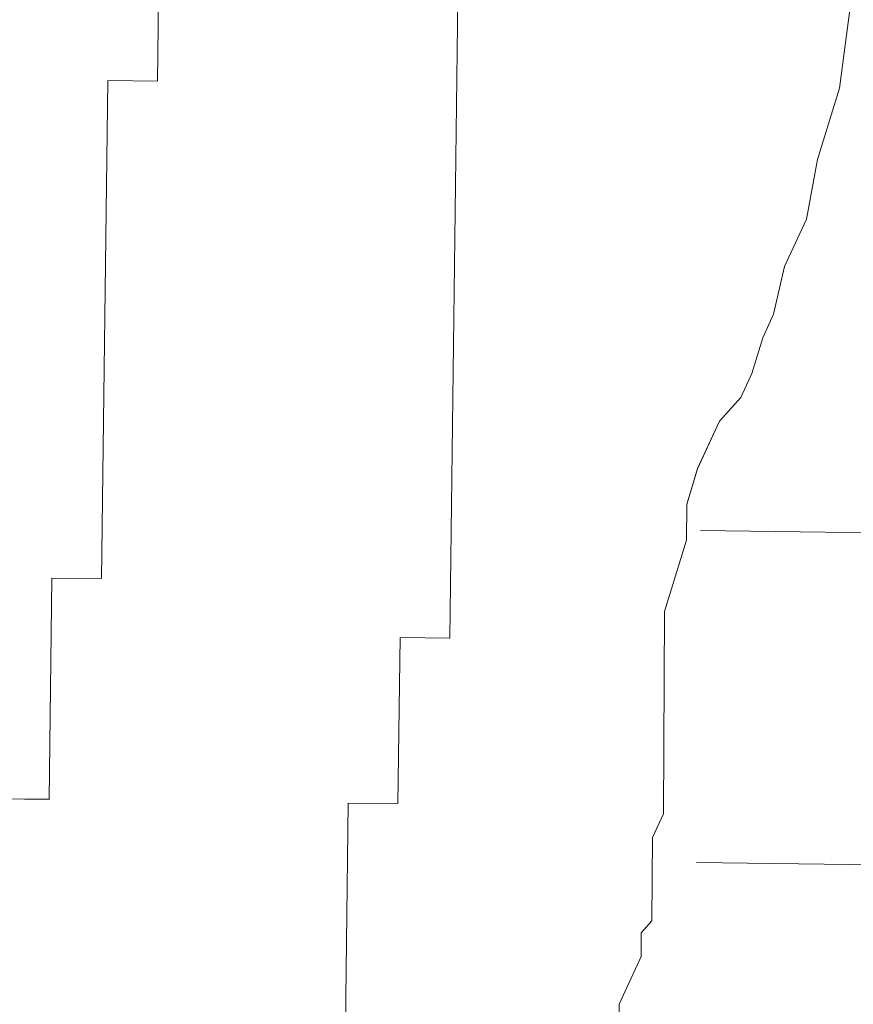
# Model space of a CAD drawing. Units: inches. Extents: x -466983 to 1020, y 324 to 318697.
# Tile 75 of 97: x 650.415 to 652.495, y 941.813 to 944.271. Entities that reach past the tile are written whole.
import ezdxf

# ---------------------------------------------------------------- set-up
doc = ezdxf.new("R2010")
doc.units = ezdxf.units.IN
doc.header["$MEASUREMENT"] = 0
doc.layers.add('A-FLOR-PATT', color=252, linetype='Continuous', lineweight=13)
doc.layers.add('A-FURN', color=8, linetype='Continuous', lineweight=18)

# ---------------------------------------------------------------- blocks, each defined once
blk = doc.blocks.new('L Shaped Sofa')
at = {"ltscale": 2}
for p, q in [((2405.1652, 744.4291), (2405.1806, 745.6886)), ((2403.9312, 745.345), (2403.9319, 745.4534)), ((2403.8323, 745.1286), (2403.9312, 745.345)), ((2403.8316, 745.0202), (2403.8323, 745.1286)), ((2403.7825, 744.9662), (2403.8316, 745.0202)), ((2403.7802, 744.5867), (2403.7825, 744.9662)), ((2399.951, 744.7447), (2403.5804, 744.7004)), ((2403.7307, 744.4785), (2403.7802, 744.5867)), ((2403.7251, 743.5568), (2403.7307, 744.4785)), ((2404.9291, 743.6761), (2404.9384, 744.4319)), ((2404.9384, 744.4319), (2405.1652, 744.4291)), ((2406.5139, 743.4048), (2406.5262, 744.4125)), ((2406.5262, 744.4125), (2406.7531, 744.4097)), ((2404.6561, 739.9002), (2404.7023, 743.6789)), ((2404.7023, 743.6789), (2404.9291, 743.6761)), ((2403.6255, 743.232), (2403.7251, 743.5568)), ((2406.2594, 741.1404), (2406.2871, 743.4076)), ((2406.2871, 743.4076), (2406.5139, 743.4048)), ((2397.4374, 743.2638), (2403.562, 743.1889)), ((2403.6245, 743.0693), (2403.6255, 743.232)), ((2403.5747, 742.9069), (2403.6245, 743.0693)), ((2403.4758, 742.6905), (2403.5747, 742.9069)), ((2403.3775, 742.5825), (2403.4758, 742.6905)), ((2403.3281, 742.4743), (2403.3775, 742.5825)), ((2403.2783, 742.3119), (2403.3281, 742.4743)), ((2403.2288, 742.2037), (2403.2783, 742.3119)), ((2403.1787, 741.9871), (2403.2288, 742.2037)), ((2403.0798, 741.7707), (2403.1787, 741.9871)), ((2403.0293, 741.4998), (2403.0798, 741.7707)), ((2402.9297, 741.175), (2403.0293, 741.4998)), ((2402.8786, 740.7957), (2402.9297, 741.175)), ((2406.0202, 740.1355), (2406.0325, 741.1431)), ((2406.0325, 741.1431), (2406.2594, 741.1404))]:
    blk.add_line(p, q, dxfattribs=at)

msp = doc.modelspace()

# ---------------------------------------------------------------- hatches: boundary and pattern name
at = {"layer": 'A-FLOR-PATT', "transparency": 33554572}
h = msp.add_hatch(dxfattribs=at)
h.set_pattern_fill('ANSI37', color=256, scale=30)
h.set_pattern_definition([(45, (-1212.4137, -290.035), (-2.6516504, 2.6516504), []), (135, (-1212.4137, -290.035), (-2.6516504, -2.6516504), [])])
h.paths.add_polyline_path([(901.8057, 1075.9377), (900.6144, 1075.9377), (900.6144, 1065.3856), (899.391, 1065.3856), (898.0911, 1065.3856), (892.8356, 1058.7098, -0.258377), (892.1875, 1058.3509), (879.9848, 1058.3509, -0.20177), (879.4382, 1058.5808), (874.0812, 1065.3856), (872.7813, 1065.3856), (871.5579, 1065.3856), (871.5579, 1075.9377), (813.8057, 1075.9377), (813.8057, 1044.7922), (832.3947, 1044.7922, -0.394795), (848.6602, 1028.5356), (848.6602, 1009.9377), (901.8057, 1009.9377), (901.8057, 1015.9377), (901.3057, 1015.9377), (871.3057, 1015.9377), (871.3057, 1017.2502), (871.3344, 1017.2502, -0.401453), (901.3057, 1045.9377), (901.8057, 1045.9377)])
edge = h.paths.add_edge_path(flags=16)
edge.add_line((847.7731, 1068.9486), (847.7731, 1073.7088))
edge.add_arc((849.2269, 1073.7088), 1.4538, 90, 180, ccw=False)
edge.add_line((849.2269, 1075.1627), (864.4921, 1075.1627))
edge.add_arc((864.4921, 1073.7088), 1.4538, 0, 90, ccw=False)
edge.add_line((865.9459, 1073.7088), (865.9459, 1069.0035))
edge.add_arc((832.6447, 1068.9761), 33.3012, -20.61234, 0.04725, ccw=False)
edge.add_ellipse((856.8595, 1058.48), major_axis=(0, 10.2131), ratio=0.6859192, start_angle=100.00884, end_angle=259.99116, ccw=False)
edge.add_arc((881.0742, 1068.9761), 33.3012, 180.04725, 200.61234, ccw=False)
h.paths.add_polyline_path([(853.1456, 1066.4815), (853.1456, 1066.4534), (853.1463, 1066.4534, 0.433107), (852.9166, 1066.6849), (852.9166, 1066.4534), (853.1456, 1066.4534), (853.1456, 1066.4815), (853.088, 1066.6122, 0.697939), (852.6995, 1066.4534), (852.7003, 1066.4534), (852.7003, 1066.4815), (852.9166, 1067.0012), (852.9166, 1066.6849, -0.396254)], flags=0)
h.paths.add_polyline_path([(861.0187, 1066.4815), (861.0187, 1066.4534), (861.0194, 1066.4534, 0.416404), (860.8024, 1066.6849), (860.8024, 1066.4534), (861.0187, 1066.4534), (861.0187, 1066.4815), (860.9672, 1066.6053, 0.713344), (860.5726, 1066.4534), (860.5734, 1066.4534), (860.5734, 1066.4815), (860.8024, 1067.0012), (860.8024, 1066.6849, -0.379973)], flags=0)
edge = h.paths.add_edge_path(flags=0)
edge.add_spline(control_points=[(861.1298, 1065.7855), (861.4661, 1065.2478), (861.6134, 1065.0161), (861.9833, 1064.3736), (862.1924, 1063.9443), (862.5614, 1063.0391), (862.7212, 1062.5633), (862.9865, 1061.5781), (863.092, 1061.0689), (863.2452, 1060.031), (863.293, 1059.5025), (863.3295, 1058.4409), (863.3181, 1057.9078), (863.2366, 1056.8518), (863.1664, 1056.3289), (862.9695, 1055.308), (862.8427, 1054.8099), (862.5365, 1053.8522), (862.3571, 1053.3927), (861.9514, 1052.5249), (861.7251, 1052.1166), (861.233, 1051.3622), (860.9672, 1051.0162), (860.4048, 1050.3949), (860.1082, 1050.1197), (859.4937, 1049.6461), (859.1758, 1049.4476), (858.5276, 1049.1299), (858.1973, 1049.0107), (857.5315, 1048.8518), (857.1959, 1048.8121), (856.5249, 1048.812), (856.1894, 1048.8515), (855.5236, 1049.0101), (855.1933, 1049.1291), (854.545, 1049.4465), (854.2271, 1049.6449), (853.6124, 1050.1183), (853.3158, 1050.3933), (852.7533, 1051.0143), (852.4874, 1051.3602), (851.9952, 1052.1144), (851.7688, 1052.5225), (851.3629, 1053.3902), (851.1834, 1053.8496), (850.877, 1054.8071), (850.7501, 1055.3051), (850.553, 1056.326), (850.4827, 1056.8488), (850.401, 1057.9048), (850.3895, 1058.4379), (850.4257, 1059.4995), (850.4734, 1060.0281), (850.6265, 1061.066), (850.7318, 1061.5753), (850.9969, 1062.5605), (851.1567, 1063.0365), (851.5254, 1063.9418), (851.7345, 1064.3712), (852.1056, 1065.0164), (852.2544, 1065.2503), (852.6082, 1065.7335)], knot_values=[3.915332, 3.915332, 3.915332, 3.915332, 4.013468, 4.013468, 4.175532, 4.175532, 4.337596, 4.337596, 4.49966, 4.49966, 4.661724, 4.661724, 4.823788, 4.823788, 4.985852, 4.985852, 5.147916, 5.147916, 5.30998, 5.30998, 5.472044, 5.472044, 5.634109, 5.634109, 5.796173, 5.796173, 5.958237, 5.958237, 6.120301, 6.120301, 6.282365, 6.282365, 6.444429, 6.444429, 6.606493, 6.606493, 6.768557, 6.768557, 6.930621, 6.930621, 7.092685, 7.092685, 7.254749, 7.254749, 7.416813, 7.416813, 7.578878, 7.578878, 7.740942, 7.740942, 7.903006, 7.903006, 8.06507, 8.06507, 8.227134, 8.227134, 8.389198, 8.389198, 8.551262, 8.551262, 8.65037, 8.65037, 8.65037, 8.65037], degree=3, periodic=0)
edge.add_line((852.6421, 1065.7855), (861.1298, 1065.7855))
edge = h.paths.add_edge_path(flags=0)
edge.add_ellipse((856.8496, 1057.7432), major_axis=(0, 7.7921), ratio=0.687861, start_angle=0, end_angle=360)
h.paths.add_polyline_path([(848.8634, 1069.3891), (848.8634, 1073.9605, -0.414214), (849.9538, 1075.0508), (863.7652, 1075.0508, -0.414214), (864.8555, 1073.9605), (864.8555, 1069.3891, -0.388936), (864.5237, 1069.027, -0.043561), (849.1953, 1069.027, -0.388936)], flags=0)
h.paths.add_polyline_path([(853.1006, 1068.1122, -1), (852.6775, 1068.1122, -1)], flags=0)
edge = h.paths.add_edge_path(flags=0)
edge.add_ellipse((856.8595, 1057.3378), major_axis=(0, 2.207), ratio=0.657164, start_angle=0, end_angle=360)
h.paths.add_polyline_path([(861.0415, 1068.1122, -1), (860.6184, 1068.1122, -1)], flags=0)
edge = h.paths.add_edge_path()
edge.add_line((573.9537, 1057.3412), (573.9537, 1075.9377))
edge.add_line((573.9537, 1075.9377), (558.7308, 1075.9377))
edge.add_line((558.7308, 1075.9377), (558.7308, 1065.3856))
edge.add_line((558.7308, 1065.3856), (557.5074, 1065.3856))
edge.add_line((557.5074, 1065.3856), (556.2075, 1065.3856))
edge.add_line((556.2075, 1065.3856), (550.952, 1058.7098))
edge.add_arc((550.3039, 1059.1155), 0.7646, 270, 327.9483, ccw=False)
edge.add_line((550.3039, 1058.3509), (538.1012, 1058.3509))
edge.add_arc((538.1012, 1059.1155), 0.7646, 224.3704, 270, ccw=False)
edge.add_line((537.5546, 1058.5808), (532.1976, 1065.3856))
edge.add_line((532.1976, 1065.3856), (530.8977, 1065.3856))
edge.add_line((530.8977, 1065.3856), (529.6743, 1065.3856))
edge.add_line((529.6743, 1065.3856), (529.6743, 1075.9377))
edge.add_line((529.6743, 1075.9377), (520.8057, 1075.9377))
edge.add_line((520.8057, 1075.9377), (520.8057, 1045.9377))
edge.add_line((520.8057, 1045.9377), (521.3057, 1045.9377))
edge.add_arc((521.3057, 1015.9377), 30, 2.50749, 90, ccw=False)
edge.add_line((551.277, 1017.2502), (551.3057, 1017.2502))
edge.add_line((551.3057, 1017.2502), (551.3057, 1015.9377))
edge.add_line((551.3057, 1015.9377), (520.8057, 1015.9377))
edge.add_line((520.8057, 1015.9377), (520.8057, 1009.9377))
edge.add_line((520.8057, 1009.9377), (559.1913, 1010.4022))
edge.add_arc((559.1913, 1011.856), 1.4538, 180, 270, ccw=False)
edge.add_line((557.7375, 1011.856), (557.7375, 1016.5613))
edge.add_arc((591.0386, 1016.5888), 33.3012, 159.38766, 180.04725, ccw=False)
edge.add_ellipse((566.8239, 1027.0848), major_axis=(0, 10.2131), ratio=0.6859192, start_angle=280.00884, end_angle=439.99116, ccw=False)
edge.add_arc((542.6091, 1016.5888), 33.3012, 0.04725, 20.61234, ccw=False)
edge.add_line((575.9103, 1016.6162), (575.9103, 1011.856))
edge.add_arc((574.4565, 1011.856), 1.4538, -90, 0, ccw=False)
edge.add_line((574.4565, 1010.4022), (608.8057, 1009.9377))
edge.add_line((608.8057, 1009.9377), (608.8057, 1041.0857))
edge.add_line((608.8057, 1041.0857), (590.2179, 1041.0857))
edge.add_arc((590.775, 1057.9074), 16.8309, 181.92775, 268.10321, ccw=False)
edge = h.paths.add_edge_path()
edge.add_ellipse((494.2443, 583.6204), major_axis=(0, 10.2131), ratio=0.6859192, start_angle=280.00884, end_angle=439.99116, ccw=False)
edge.add_arc((470.0296, 573.1243), 33.3012, 0.04725, 20.61234, ccw=False)
edge.add_line((503.3307, 573.1518), (503.3307, 568.3916))
edge.add_arc((501.8769, 568.3916), 1.4538, -90, 0, ccw=False)
edge.add_line((501.8769, 566.9377), (539.8057, 566.9377))
edge.add_line((539.8057, 566.9377), (539.8057, 572.9377))
edge.add_line((539.8057, 572.9377), (539.3057, 572.9377))
edge.add_line((539.3057, 572.9377), (509.3057, 572.9377))
edge.add_line((509.3057, 572.9377), (509.3057, 574.2502))
edge.add_line((509.3057, 574.2502), (509.3344, 574.2502))
edge.add_arc((539.3057, 572.9377), 30, 90, 177.49251, ccw=False)
edge.add_line((539.3057, 602.9377), (539.8057, 602.9377))
edge.add_line((539.8057, 602.9377), (539.8057, 626.9377))
edge.add_line((539.8057, 626.9377), (531.7718, 626.9377))
edge.add_line((531.7718, 626.9377), (531.7718, 616.3856))
edge.add_line((531.7718, 616.3856), (530.5484, 616.3856))
edge.add_line((530.5484, 616.3856), (529.2485, 616.3856))
edge.add_line((529.2485, 616.3856), (523.7105, 609.3509))
edge.add_line((523.7105, 609.3509), (510.7766, 609.3509))
edge.add_line((510.7766, 609.3509), (505.2386, 616.3856))
edge.add_line((505.2386, 616.3856), (503.9387, 616.3856))
edge.add_line((503.9387, 616.3856), (502.7153, 616.3856))
edge.add_line((502.7153, 616.3856), (502.7153, 626.9377))
edge.add_line((502.7153, 626.9377), (481.6983, 626.9377))
edge.add_line((481.6983, 626.9377), (481.6983, 610.995))
edge.add_arc((467.2703, 611.4728), 14.4359, 271.92775, 358.10321, ccw=False)
edge.add_line((467.7559, 597.0451), (451.8057, 597.0451))
edge.add_line((451.8057, 597.0451), (451.8057, 584.4035))
edge.add_line((451.8057, 584.4035), (451.8057, 566.9377))
edge.add_line((451.8057, 566.9377), (486.6117, 566.9377))
edge.add_arc((486.6117, 568.3916), 1.4538, 180, 270, ccw=False)
edge.add_line((485.1579, 568.3916), (485.1579, 573.0969))
edge.add_arc((518.4591, 573.1243), 33.3012, 159.38766, 180.04725, ccw=False)
h.paths.add_polyline_path([(836.2609, 1020.7328), (879.8898, 1020.7328), (879.8898, 1039.3902), (836.2609, 1039.3902)], flags=25)
h.paths.add_polyline_path([(549.9851, 1036.7492), (593.614, 1036.7492), (593.614, 1055.4065), (549.9851, 1055.4065)], flags=24)
h.paths.add_polyline_path([(475.123, 595.5959), (518.752, 595.5959), (518.752, 614.2532), (475.123, 614.2532)], flags=24)
h = msp.add_hatch(dxfattribs=at)
h.set_pattern_fill('ANSI37', color=256, scale=20)
h.set_pattern_definition([(45, (-1212.4137, -290.035), (-1.767767, 1.767767), []), (135, (-1212.4137, -290.035), (-1.767767, -1.767767), [])])
h.paths.add_polyline_path([(809.8057, 870.9377), (809.8057, 888.1519), (806.9985, 888.1519), (802.6624, 888.1519), (789.3832, 888.1519), (786.2846, 888.1519, -0.414214), (785.4991, 888.9374), (785.4991, 900.1959), (785.4991, 908.4696, -0.414214), (786.8082, 909.7787, -0.414214), (785.4991, 911.0878), (785.4991, 929.1015, -0.414214), (786.8082, 930.4106, -0.414214), (785.4991, 931.7197), (785.4991, 931.9039, -0.414214), (784.19, 930.5948), (766.7223, 930.5948, -0.412359), (765.4132, 931.8956, -0.413741), (764.1145, 930.5782), (744.5781, 930.422, -0.416556), (743.7864, 931.2075), (743.7864, 933.5153), (742.2154, 933.5153), (742.2154, 952.024, -0.001344), (743.7864, 952.1998), (743.7864, 953.9377), (678.5915, 953.9377), (678.5915, 951.1305), (678.5915, 946.7945), (678.5915, 933.5153), (678.5915, 930.4166, -0.414214), (677.806, 929.6312), (666.5475, 929.6312), (658.2738, 929.6312, -0.414214), (656.9647, 930.9403, -0.414214), (655.6556, 929.6312), (637.6419, 929.6312, -0.414214), (636.3328, 930.9403, -0.414214), (635.0237, 929.6312), (634.8395, 929.6312, -0.414214), (636.1486, 928.322), (636.1486, 910.8544, -0.412359), (634.8478, 909.5452, -0.413741), (636.1653, 908.2466), (636.3214, 888.7102, -0.416556), (635.5359, 887.9184), (633.2281, 887.9184), (633.2281, 886.3475), (614.7194, 886.3475, -0.001344), (614.5436, 887.9184), (612.8057, 887.9184), (612.8057, 834.9377), (612.8057, 752.9377), (612.8057, 748.9377), (612.8057, 697.9377), (654.8057, 697.9377), (654.8057, 701.9377), (715.8057, 701.9377), (715.8057, 737.4353), (774.2918, 737.4353), (774.2918, 795.9377), (809.8057, 795.9377)])
h.paths.add_polyline_path([(679.2761, 849.5757, 0.102523), (682.1475, 849.2608, -0.080461), (694.5428, 849.7725, -0.283899), (694.4822, 849.0082, 0.136605), (694.4068, 848.8103, -0.030441), (694.5428, 846.8929), (694.5428, 842.6198), (694.5428, 838.3466, -0.028219), (694.4246, 836.5684), (694.425, 836.5684, 0.196187), (694.4456, 836.2708, -0.302897), (694.5428, 835.467, -0.080461), (682.1475, 835.9787, 0.102523), (679.2761, 835.6638, -0.58611), (678.6457, 836.0169), (678.6457, 849.2227, -0.58611)], flags=16)
h.paths.add_polyline_path([(679.5173, 848.6515, 0.699597), (679.476, 848.6342, 1.20716), (679.1935, 848.7422, 0.010621)], flags=0)
h.paths.add_polyline_path([(679.4923, 836.5608, -0.013798), (679.9178, 836.6594, -0.071703), (682.8533, 837.1434, -0.165743), (682.1665, 839.1006), (682.1665, 842.6094), (682.1665, 846.0603, -0.240616), (683.4733, 848.6767, -0.068263), (693.9295, 849.0082), (693.7875, 848.7083), (693.7875, 849.0228, 0.067332), (683.4733, 848.6767, 0.240616), (682.1665, 846.0603), (682.1665, 842.6094), (682.1665, 839.1006, 0.23459), (683.461, 836.5513, 0.068093), (693.7875, 836.1955), (693.7875, 836.5104), (693.9296, 836.2102, -0.077215), (682.2421, 836.7815, 0.086627), (679.5283, 836.5701, -0.628402), (679.5029, 836.5735), (679.5029, 836.6071, 0.910458)], flags=0)
h.paths.add_polyline_path([(679.476, 848.6364), (679.2069, 848.647), (679.2069, 836.5718, 0.913566), (679.3645, 836.5861), (679.476, 836.5824)], flags=0)
h.paths.add_polyline_path([(679.2761, 829.8604, 0.102523), (682.1475, 829.5455, -0.080461), (694.5428, 830.0572, -0.283899), (694.4822, 829.2929, 0.136605), (694.4068, 829.095, -0.030441), (694.5428, 827.1776), (694.5428, 822.9045), (694.5428, 818.6314, -0.028219), (694.4246, 816.8531), (694.425, 816.8532, 0.196187), (694.4456, 816.5555, -0.302897), (694.5428, 815.7517, -0.080461), (682.1475, 816.2635, 0.102523), (679.2761, 815.9485, -0.58611), (678.6457, 816.3016), (678.6457, 829.5074, -0.58611)], flags=16)
h.paths.add_polyline_path([(679.5173, 828.9362, 0.699597), (679.476, 828.9189, 1.20716), (679.1935, 829.0269, 0.010621)], flags=0)
h.paths.add_polyline_path([(679.4923, 816.8456, -0.013798), (679.9178, 816.9441, -0.071703), (682.8533, 817.4281, -0.165743), (682.1665, 819.3853), (682.1665, 822.8941), (682.1665, 826.345, -0.240616), (683.4733, 828.9614, -0.068263), (693.9295, 829.2929), (693.7875, 828.9931), (693.7875, 829.3076, 0.067332), (683.4733, 828.9614, 0.240616), (682.1665, 826.345), (682.1665, 822.8941), (682.1665, 819.3853, 0.23459), (683.461, 816.836, 0.068093), (693.7875, 816.4802), (693.7875, 816.7952), (693.9296, 816.4949, -0.077215), (682.2421, 817.0662, 0.086627), (679.5283, 816.8549, -0.628402), (679.5029, 816.8582), (679.5029, 816.8918, 0.910458)], flags=0)
h.paths.add_polyline_path([(679.476, 828.9211), (679.2069, 828.9317), (679.2069, 816.8565, 0.913566), (679.3645, 816.8708), (679.476, 816.8671)], flags=0)
h.paths.add_polyline_path([(679.2761, 810.1451, 0.102523), (682.1475, 809.8302, -0.080461), (694.5428, 810.342, -0.3023), (694.4466, 809.5394, 0.10023), (694.4058, 809.3878, -0.03057), (694.5428, 807.4623), (694.5428, 803.1892), (694.5428, 798.9161, -0.03057), (694.4058, 796.9906, 0.10023), (694.4466, 796.839, -0.3023), (694.5428, 796.0365, -0.080461), (682.1475, 796.5482, 0.102523), (679.2761, 796.2333, -0.58611), (678.6457, 796.5863), (678.6457, 809.7921, -0.58611)], flags=16)
h.paths.add_polyline_path([(679.5173, 809.2417, 0.699597), (679.476, 809.2244, 1.20716), (679.1935, 809.3324, 0.010621)], flags=0)
h.paths.add_polyline_path([(679.4923, 797.151, -0.013798), (679.9178, 797.2496, -0.071703), (682.8533, 797.7336, -0.165743), (682.1665, 799.6908), (682.1665, 803.1996), (682.1665, 806.6505, -0.239349), (683.461, 809.2577, -0.072465), (694.4468, 809.5405, 0.197932), (694.425, 809.2405), (693.7875, 809.2985), (693.7875, 809.6135, 0.068093), (683.461, 809.2577, 0.239349), (682.1665, 806.6505), (682.1665, 803.1996), (682.1665, 799.6908, 0.235854), (683.4733, 797.1323, 0.067332), (693.7875, 796.7861), (693.7875, 797.1006), (694.425, 797.1586, 0.197932), (694.4468, 796.8586, -0.080419), (682.1557, 797.3795, 0.083867), (679.5283, 797.1603, -0.628402), (679.5029, 797.1637), (679.5029, 797.1973, 0.910458)], flags=0)
h.paths.add_polyline_path([(679.2069, 809.2372), (679.2069, 797.162, 0.913566), (679.3645, 797.1763), (679.476, 797.1726), (679.476, 809.2266)], flags=0)
h.paths.add_polyline_path([(695.3643, 853.2989), (728.2231, 853.2989), (728.2231, 771.1519), (695.3643, 771.1519)], flags=16)
h.paths.add_polyline_path([(696.0215, 852.6417), (727.5659, 852.6417), (727.5659, 771.809), (696.0215, 771.809)], flags=0)
h.paths.add_polyline_path([(679.2761, 788.7869, 0.102523), (682.1475, 788.472, -0.080461), (694.5428, 788.9837, -0.3023), (694.4466, 788.1812, 0.10023), (694.4058, 788.0296, -0.03057), (694.5428, 786.1041), (694.5428, 781.831), (694.5428, 777.5578, -0.03057), (694.4058, 775.6323, 0.10023), (694.4466, 775.4808, -0.3023), (694.5428, 774.6782, -0.080461), (682.1475, 775.19, 0.102523), (679.2761, 774.875, -0.58611), (678.6457, 775.2281), (678.6457, 788.4339, -0.58611)], flags=16)
h.paths.add_polyline_path([(679.5173, 787.8834, 0.699597), (679.476, 787.8662, 1.20716), (679.1935, 787.9742, 0.010621)], flags=0)
h.paths.add_polyline_path([(679.4923, 775.7928, -0.013798), (679.9178, 775.8914, -0.071703), (682.8533, 776.3753, -0.165743), (682.1665, 778.3325), (682.1665, 781.8414), (682.1665, 785.2922, -0.239349), (683.461, 787.8995, -0.072465), (694.4468, 788.1823, 0.197932), (694.425, 787.8823), (693.7875, 787.9403), (693.7875, 788.2553, 0.068093), (683.461, 787.8995, 0.239349), (682.1665, 785.2922), (682.1665, 781.8414), (682.1665, 778.3325, 0.235854), (683.4733, 775.7741, 0.067332), (693.7875, 775.4279), (693.7875, 775.7424), (694.425, 775.8004, 0.197932), (694.4468, 775.5004, -0.080419), (682.1557, 776.0212, 0.083867), (679.5283, 775.8021, -0.628402), (679.5029, 775.8054), (679.5029, 775.8391, 0.910458)], flags=0)
h.paths.add_polyline_path([(679.2069, 787.8789), (679.2069, 775.8038, 0.913566), (679.3645, 775.818), (679.476, 775.8144), (679.476, 787.8684)], flags=0)
h.paths.add_polyline_path([(704.641, 854.1204, -0.080461), (705.1527, 866.5157, 0.102523), (704.8378, 869.3871, -0.58611), (705.1908, 870.0174), (718.3966, 870.0174, -0.58611), (718.7496, 869.3871, 0.102523), (718.4347, 866.5157, -0.080461), (718.9465, 854.1204, -0.3023), (718.1439, 854.2166, 0.10023), (717.9924, 854.2574, -0.03057), (716.0668, 854.1204), (711.7937, 854.1204), (707.5206, 854.1204, -0.03057), (705.5951, 854.2574, 0.10023), (705.4435, 854.2166, -0.3023)], flags=16)
h.paths.add_polyline_path([(717.8462, 869.1459, 0.699597), (717.8289, 869.1872, 1.20716), (717.9369, 869.4697, 0.010621)], flags=0)
h.paths.add_polyline_path([(705.4631, 854.2164, -0.080419), (705.984, 866.5074, 0.083867), (705.7648, 869.1349, -0.628402), (705.7682, 869.1603), (705.8018, 869.1603, 0.910458), (705.7555, 869.1709, -0.013798), (705.8541, 868.7454, -0.071703), (706.3381, 865.8099, -0.165743), (708.2953, 866.4967), (711.8041, 866.4967), (715.255, 866.4967, -0.239349), (717.8622, 865.2022, -0.072465), (718.145, 854.2164, 0.197932), (717.845, 854.2382), (717.903, 854.8757), (718.218, 854.8757, 0.068093), (717.8622, 865.2022, 0.239349), (715.255, 866.4967), (711.8041, 866.4967), (708.2953, 866.4967, 0.235854), (705.7368, 865.1898, 0.067332), (705.3906, 854.8757), (705.7051, 854.8757), (705.7631, 854.2382, 0.197932)], flags=16)
h.paths.add_polyline_path([(705.7665, 869.4563, 0.913566), (705.7808, 869.2987), (705.7771, 869.1872), (717.8311, 869.1872), (717.8417, 869.4563)], flags=0)
h.paths.add_polyline_path([(729.0446, 842.6198), (729.0446, 846.8929, -0.03057), (729.1817, 848.8184, 0.10023), (729.1408, 848.9699, -0.3023), (729.0446, 849.7725, -0.080461), (741.4399, 849.2608, 0.102523), (744.3113, 849.5757, -0.58611), (744.9417, 849.2227), (744.9417, 836.0169, -0.58611), (744.3113, 835.6638, 0.102523), (741.4399, 835.9787, -0.080461), (729.0446, 835.467, -0.3023), (729.1408, 836.2696, 0.10023), (729.1817, 836.4211, -0.03057), (729.0446, 838.3466)], flags=16)
h.paths.add_polyline_path([(744.1115, 836.5846, 1.20716), (744.3939, 836.4766, 0.010621), (744.0701, 836.5673, 0.699597)], flags=0)
h.paths.add_polyline_path([(729.1407, 836.2684, 0.197932), (729.1624, 836.5684), (729.7999, 836.5104), (729.7999, 836.1955, 0.068093), (740.1264, 836.5513, 0.239349), (741.4209, 839.1585), (741.4209, 842.6094), (741.4209, 846.1182, 0.235854), (740.1141, 848.6767, 0.067332), (729.7999, 849.0228), (729.7999, 848.7083), (729.1624, 848.6503, 0.197932), (729.1407, 848.9504, -0.080419), (741.4317, 848.4295, 0.083867), (744.0591, 848.6486, -0.628402), (744.0845, 848.6453), (744.0845, 848.6117, 0.910458), (744.0951, 848.6579, -0.013798), (743.6696, 848.5594, -0.071703), (740.7341, 848.0754, -0.165743), (741.4209, 846.1182), (741.4209, 842.6094), (741.4209, 839.1585, -0.239349), (740.1264, 836.5513, -0.072465)], flags=0)
h.paths.add_polyline_path([(729.0446, 830.0572, -0.080461), (741.4399, 829.5455, 0.102523), (744.3113, 829.8604, -0.58611), (744.9417, 829.5074), (744.9417, 816.3016, -0.58611), (744.3113, 815.9485, 0.102523), (741.4399, 816.2635, -0.080461), (729.0446, 815.7517, -0.3023), (729.1408, 816.5543, 0.10023), (729.1817, 816.7058, -0.03057), (729.0446, 818.6314), (729.0446, 822.9045), (729.0446, 827.1776, -0.03057), (729.1817, 829.1031, 0.10023), (729.1408, 829.2547, -0.3023)], flags=16)
h.paths.add_polyline_path([(744.1115, 816.8693, 1.20716), (744.3939, 816.7613, 0.010621), (744.0701, 816.852, 0.699597)], flags=0)
h.paths.add_polyline_path([(729.1407, 829.2351, -0.080419), (741.4317, 828.7142, 0.083867), (744.0591, 828.9334, -0.628402), (744.0845, 828.93), (744.0845, 828.8964, 0.910458), (744.0951, 828.9427, -0.013798), (743.6696, 828.8441, -0.071703), (740.7341, 828.3601, -0.165743), (741.4209, 826.4029), (741.4209, 822.8941), (741.4209, 819.4432, -0.239349), (740.1264, 816.836, -0.072465), (729.1407, 816.5531, 0.197932), (729.1624, 816.8532), (729.7999, 816.7952), (729.7999, 816.4802, 0.068093), (740.1264, 816.836, 0.239349), (741.4209, 819.4432), (741.4209, 822.8941), (741.4209, 826.4029, 0.235854), (740.1141, 828.9614, 0.067332), (729.7999, 829.3076), (729.7999, 828.9931), (729.1624, 828.9351, 0.197932)], flags=16)
h.paths.add_polyline_path([(729.0446, 810.342, -0.080461), (741.4399, 809.8302, 0.102523), (744.3113, 810.1451, -0.58611), (744.9417, 809.7921), (744.9417, 796.5863, -0.58611), (744.3113, 796.2333, 0.102523), (741.4399, 796.5482, -0.080461), (729.0446, 796.0365, -0.283899), (729.1052, 796.8007, 0.136605), (729.1806, 796.9987, -0.030441), (729.0446, 798.9161), (729.0446, 803.1892), (729.0446, 807.4623, -0.028219), (729.1628, 809.2406), (729.1624, 809.2405, 0.196187), (729.1418, 809.5382, -0.302897)], flags=16)
h.paths.add_polyline_path([(744.1115, 797.1748, 1.20716), (744.3939, 797.0668, 0.010621), (744.0701, 797.1575, 0.699597)], flags=0)
h.paths.add_polyline_path([(741.3453, 809.0275, 0.086627), (744.0591, 809.2388, -0.628402), (744.0845, 809.2355), (744.0845, 809.2019, 0.910458), (744.0951, 809.2481, -0.013798), (743.6696, 809.1496, -0.071703), (740.7341, 808.6656, -0.165743), (741.4209, 806.7084), (741.4209, 803.1996), (741.4209, 799.7487, -0.240616), (740.1141, 797.1323, -0.068263), (729.658, 796.8008), (729.7999, 797.1006), (729.7999, 796.7861, 0.067332), (740.1141, 797.1323, 0.240616), (741.4209, 799.7487), (741.4209, 803.1996), (741.4209, 806.7084, 0.23459), (740.1264, 809.2577, 0.068093), (729.7999, 809.6135), (729.7999, 809.2985), (729.6578, 809.5988, -0.077215)], flags=0)
h.paths.add_polyline_path([(704.641, 770.3304, -0.283899), (705.4053, 770.2697, 0.136605), (705.6032, 770.1944, -0.030441), (707.5206, 770.3304), (711.7937, 770.3304), (716.0668, 770.3304, -0.028219), (717.8451, 770.2122), (717.845, 770.2126, 0.196187), (718.1427, 770.2331, -0.302897), (718.9465, 770.3304, -0.080461), (718.4347, 757.9351, 0.102523), (718.7496, 755.0637, -0.58611), (718.3966, 754.4333), (705.1908, 754.4333, -0.58611), (704.8378, 755.0637, 0.102523), (705.1527, 757.9351, -0.080461)], flags=16)
h.paths.add_polyline_path([(705.762, 755.3048, 0.699597), (705.7793, 755.2635, 1.20716), (705.6713, 754.9811, 0.010621)], flags=0)
h.paths.add_polyline_path([(705.4053, 769.717), (705.7051, 769.5751), (705.3906, 769.5751, 0.067332), (705.7368, 759.2609, 0.240616), (708.3532, 757.954), (711.8041, 757.954), (715.3129, 757.954, 0.23459), (717.8622, 759.2485, 0.068093), (718.218, 769.5751), (717.903, 769.5751), (718.2033, 769.7172, -0.077215), (717.632, 758.0297, 0.086627), (717.8433, 755.3159, -0.628402), (717.84, 755.2904), (717.8064, 755.2904, 0.910458), (717.8526, 755.2799, -0.013798), (717.7541, 755.7053, -0.071703), (717.2701, 758.6409, -0.165743), (715.3129, 757.954), (711.8041, 757.954), (708.3532, 757.954, -0.240616), (705.7368, 759.2609, -0.068263)], flags=0)
h.paths.add_polyline_path([(729.0446, 788.9837, -0.080461), (741.4399, 788.472, 0.102523), (744.3113, 788.7869, -0.58611), (744.9417, 788.4339), (744.9417, 775.2281, -0.58611), (744.3113, 774.875, 0.102523), (741.4399, 775.19, -0.080461), (729.0446, 774.6782, -0.283899), (729.1052, 775.4425, 0.136605), (729.1806, 775.6405, -0.030441), (729.0446, 777.5578), (729.0446, 781.831), (729.0446, 786.1041, -0.028219), (729.1628, 787.8823), (729.1624, 787.8823, 0.196187), (729.1418, 788.1799, -0.302897)], flags=16)
h.paths.add_polyline_path([(744.1115, 775.8165, 1.20716), (744.3939, 775.7086, 0.010621), (744.0701, 775.7993, 0.699597)], flags=0)
h.paths.add_polyline_path([(741.3453, 787.6692, 0.086627), (744.0591, 787.8806, -0.628402), (744.0845, 787.8773), (744.0845, 787.8437, 0.910458), (744.0951, 787.8899, -0.013798), (743.6696, 787.7913, -0.071703), (740.7341, 787.3074, -0.165743), (741.4209, 785.3502), (741.4209, 781.8414), (741.4209, 778.3905, -0.240616), (740.1141, 775.7741, -0.068263), (729.658, 775.4425), (729.7999, 775.7424), (729.7999, 775.4279, 0.067332), (740.1141, 775.7741, 0.240616), (741.4209, 778.3905), (741.4209, 781.8414), (741.4209, 785.3502, 0.23459), (740.1264, 787.8995, 0.068093), (729.7999, 788.2553), (729.7999, 787.9403), (729.6578, 788.2405, -0.077215)], flags=0)
h.paths.add_polyline_path([(744.1115, 848.6364), (744.1115, 836.5824), (744.3805, 836.5718), (744.3805, 848.647, 0.913566), (744.2229, 848.6327)], flags=0)
h.paths.add_polyline_path([(744.2229, 828.9174), (744.1115, 828.9211), (744.1115, 816.8671), (744.3805, 816.8565), (744.3805, 828.9317, 0.913566)], flags=0)
h.paths.add_polyline_path([(717.8311, 755.2635), (705.7771, 755.2635), (705.7665, 754.9945), (717.8417, 754.9945, 0.913566), (717.8274, 755.1521)], flags=0)
h.paths.add_polyline_path([(744.2229, 809.2229), (744.1115, 809.2266), (744.1115, 797.1726), (744.3805, 797.162), (744.3805, 809.2372, 0.913566)], flags=0)
h.paths.add_polyline_path([(744.1115, 787.8684), (744.1115, 775.8144), (744.3805, 775.8038), (744.3805, 787.8789, 0.913566), (744.2229, 787.8647)], flags=0)
h.paths.add_polyline_path([(678.8774, 877.1228), (737.6127, 877.1228), (737.6127, 899.5116), (678.8774, 899.5116)], flags=24)

# ---------------------------------------------------------------- linework, layer by layer
at = {"layer": 'A-FURN', "ltscale": 2}
for p, q in [((651.5133, 944.7985), (651.488, 942.727)), ((651.5133, 944.7985), (651.488, 942.727)), ((651.5133, 944.7985), (651.488, 942.727)), ((651.5133, 944.7985), (651.488, 942.727)), ((651.5133, 944.7985), (651.488, 942.727)), ((651.5133, 944.7985), (651.488, 942.727)), ((650.7655, 944.6696), (650.7588, 944.1171)), ((650.7655, 944.6696), (650.7588, 944.1171)), ((650.7655, 944.6696), (650.7588, 944.1171)), ((650.7655, 944.6696), (650.7588, 944.1171)), ((650.7655, 944.6696), (650.7588, 944.1171)), ((650.7655, 944.6696), (650.7588, 944.1171)), ((652.4878, 944.3076), (652.4598, 944.0997)), ((652.4878, 944.3076), (652.4598, 944.0997)), ((652.4878, 944.3076), (652.4598, 944.0997)), ((652.4878, 944.3076), (652.4598, 944.0997)), ((652.4878, 944.3076), (652.4598, 944.0997)), ((652.4878, 944.3076), (652.4598, 944.0997)), ((650.6344, 944.1187), (650.6192, 942.8757)), ((650.6344, 944.1187), (650.6192, 942.8757)), ((650.6344, 944.1187), (650.6192, 942.8757)), ((650.6344, 944.1187), (650.6192, 942.8757)), ((650.6344, 944.1187), (650.6192, 942.8757)), ((650.6344, 944.1187), (650.6192, 942.8757)), ((650.7588, 944.1171), (650.6344, 944.1187)), ((650.7588, 944.1171), (650.6344, 944.1187)), ((650.7588, 944.1171), (650.6344, 944.1187)), ((650.7588, 944.1171), (650.6344, 944.1187)), ((650.7588, 944.1171), (650.6344, 944.1187)), ((650.7588, 944.1171), (650.6344, 944.1187)), ((652.4598, 944.0997), (652.4052, 943.9216)), ((652.4598, 944.0997), (652.4052, 943.9216)), ((652.4598, 944.0997), (652.4052, 943.9216)), ((652.4598, 944.0997), (652.4052, 943.9216)), ((652.4598, 944.0997), (652.4052, 943.9216)), ((652.4598, 944.0997), (652.4052, 943.9216)), ((652.4052, 943.9216), (652.3775, 943.7731)), ((652.4052, 943.9216), (652.3775, 943.7731)), ((652.4052, 943.9216), (652.3775, 943.7731)), ((652.4052, 943.9216), (652.3775, 943.7731)), ((652.4052, 943.9216), (652.3775, 943.7731)), ((652.4052, 943.9216), (652.3775, 943.7731)), ((652.3775, 943.7731), (652.3233, 943.6545)), ((652.3775, 943.7731), (652.3233, 943.6545)), ((652.3775, 943.7731), (652.3233, 943.6545)), ((652.3775, 943.7731), (652.3233, 943.6545)), ((652.3775, 943.7731), (652.3233, 943.6545)), ((652.3775, 943.7731), (652.3233, 943.6545)), ((652.3233, 943.6545), (652.2958, 943.5357)), ((652.3233, 943.6545), (652.2958, 943.5357)), ((652.3233, 943.6545), (652.2958, 943.5357)), ((652.3233, 943.6545), (652.2958, 943.5357)), ((652.3233, 943.6545), (652.2958, 943.5357)), ((652.3233, 943.6545), (652.2958, 943.5357)), ((652.2958, 943.5357), (652.2687, 943.4764)), ((652.2958, 943.5357), (652.2687, 943.4764)), ((652.2958, 943.5357), (652.2687, 943.4764)), ((652.2958, 943.5357), (652.2687, 943.4764)), ((652.2958, 943.5357), (652.2687, 943.4764)), ((652.2958, 943.5357), (652.2687, 943.4764)), ((652.2687, 943.4764), (652.2414, 943.3874)), ((652.2687, 943.4764), (652.2414, 943.3874)), ((652.2687, 943.4764), (652.2414, 943.3874)), ((652.2687, 943.4764), (652.2414, 943.3874)), ((652.2687, 943.4764), (652.2414, 943.3874)), ((652.2687, 943.4764), (652.2414, 943.3874)), ((652.2414, 943.3874), (652.2143, 943.3281)), ((652.2414, 943.3874), (652.2143, 943.3281)), ((652.2414, 943.3874), (652.2143, 943.3281)), ((652.2414, 943.3874), (652.2143, 943.3281)), ((652.2414, 943.3874), (652.2143, 943.3281)), ((652.2414, 943.3874), (652.2143, 943.3281)), ((652.2143, 943.3281), (652.1604, 943.2689)), ((652.2143, 943.3281), (652.1604, 943.2689)), ((652.2143, 943.3281), (652.1604, 943.2689)), ((652.2143, 943.3281), (652.1604, 943.2689)), ((652.2143, 943.3281), (652.1604, 943.2689)), ((652.2143, 943.3281), (652.1604, 943.2689)), ((652.1604, 943.2689), (652.1062, 943.1502)), ((652.1604, 943.2689), (652.1062, 943.1502)), ((652.1604, 943.2689), (652.1062, 943.1502)), ((652.1604, 943.2689), (652.1062, 943.1502)), ((652.1604, 943.2689), (652.1062, 943.1502)), ((652.1604, 943.2689), (652.1062, 943.1502)), ((652.1062, 943.1502), (652.0789, 943.0612)), ((652.1062, 943.1502), (652.0789, 943.0612)), ((652.1062, 943.1502), (652.0789, 943.0612)), ((652.1062, 943.1502), (652.0789, 943.0612)), ((652.1062, 943.1502), (652.0789, 943.0612)), ((652.1062, 943.1502), (652.0789, 943.0612)), ((652.0789, 943.0612), (652.0784, 942.972)), ((652.0789, 943.0612), (652.0784, 942.972)), ((652.0789, 943.0612), (652.0784, 942.972)), ((652.0789, 943.0612), (652.0784, 942.972)), ((652.0789, 943.0612), (652.0784, 942.972)), ((652.0789, 943.0612), (652.0784, 942.972)), ((655.4708, 942.9546), (652.1132, 942.9956)), ((655.4708, 942.9546), (652.1132, 942.9956)), ((655.4708, 942.9546), (652.1132, 942.9956)), ((655.4708, 942.9546), (652.1132, 942.9956)), ((655.4708, 942.9546), (652.1132, 942.9956)), ((655.4708, 942.9546), (652.1132, 942.9956)), ((652.0784, 942.972), (652.0238, 942.7939)), ((652.0784, 942.972), (652.0238, 942.7939)), ((652.0784, 942.972), (652.0238, 942.7939)), ((652.0784, 942.972), (652.0238, 942.7939)), ((652.0784, 942.972), (652.0238, 942.7939)), ((652.0784, 942.972), (652.0238, 942.7939)), ((650.4949, 942.8773), (650.4881, 942.3249)), ((650.4949, 942.8773), (650.4881, 942.3249)), ((650.4949, 942.8773), (650.4881, 942.3249)), ((650.4949, 942.8773), (650.4881, 942.3249)), ((650.4949, 942.8773), (650.4881, 942.3249)), ((650.4949, 942.8773), (650.4881, 942.3249)), ((650.6192, 942.8757), (650.4949, 942.8773)), ((650.6192, 942.8757), (650.4949, 942.8773)), ((650.6192, 942.8757), (650.4949, 942.8773)), ((650.6192, 942.8757), (650.4949, 942.8773)), ((650.6192, 942.8757), (650.4949, 942.8773)), ((650.6192, 942.8757), (650.4949, 942.8773)), ((652.0238, 942.7939), (652.0207, 942.2887)), ((652.0238, 942.7939), (652.0207, 942.2887)), ((652.0238, 942.7939), (652.0207, 942.2887)), ((652.0238, 942.7939), (652.0207, 942.2887)), ((652.0238, 942.7939), (652.0207, 942.2887)), ((652.0238, 942.7939), (652.0207, 942.2887)), ((651.3637, 942.7285), (651.3586, 942.3142)), ((651.3637, 942.7285), (651.3586, 942.3142)), ((651.3637, 942.7285), (651.3586, 942.3142)), ((651.3637, 942.7285), (651.3586, 942.3142)), ((651.3637, 942.7285), (651.3586, 942.3142)), ((651.3637, 942.7285), (651.3586, 942.3142)), ((651.488, 942.727), (651.3637, 942.7285)), ((651.488, 942.727), (651.3637, 942.7285)), ((651.488, 942.727), (651.3637, 942.7285)), ((651.488, 942.727), (651.3637, 942.7285)), ((651.488, 942.727), (651.3637, 942.7285)), ((651.488, 942.727), (651.3637, 942.7285)), ((650.4881, 942.3249), (650.3638, 942.3264)), ((650.4881, 942.3249), (650.3638, 942.3264)), ((650.4881, 942.3249), (650.3638, 942.3264)), ((650.4881, 942.3249), (650.3638, 942.3264)), ((650.4881, 942.3249), (650.3638, 942.3264)), ((650.4881, 942.3249), (650.3638, 942.3264)), ((651.2343, 942.3157), (651.2258, 941.6252)), ((651.2343, 942.3157), (651.2258, 941.6252)), ((651.2343, 942.3157), (651.2258, 941.6252)), ((651.2343, 942.3157), (651.2258, 941.6252)), ((651.2343, 942.3157), (651.2258, 941.6252)), ((651.2343, 942.3157), (651.2258, 941.6252)), ((651.3586, 942.3142), (651.2343, 942.3157)), ((651.3586, 942.3142), (651.2343, 942.3157)), ((651.3586, 942.3142), (651.2343, 942.3157)), ((651.3586, 942.3142), (651.2343, 942.3157)), ((651.3586, 942.3142), (651.2343, 942.3157)), ((651.3586, 942.3142), (651.2343, 942.3157)), ((652.0207, 942.2887), (651.9936, 942.2293)), ((652.0207, 942.2887), (651.9936, 942.2293)), ((652.0207, 942.2887), (651.9936, 942.2293)), ((652.0207, 942.2887), (651.9936, 942.2293)), ((652.0207, 942.2887), (651.9936, 942.2293)), ((652.0207, 942.2887), (651.9936, 942.2293)), ((651.9936, 942.2293), (651.9923, 942.0213)), ((651.9936, 942.2293), (651.9923, 942.0213)), ((651.9936, 942.2293), (651.9923, 942.0213)), ((651.9936, 942.2293), (651.9923, 942.0213)), ((651.9936, 942.2293), (651.9923, 942.0213)), ((651.9936, 942.2293), (651.9923, 942.0213)), ((654.0927, 942.1427), (652.1031, 942.167)), ((654.0927, 942.1427), (652.1031, 942.167)), ((654.0927, 942.1427), (652.1031, 942.167)), ((654.0927, 942.1427), (652.1031, 942.167)), ((654.0927, 942.1427), (652.1031, 942.167)), ((654.0927, 942.1427), (652.1031, 942.167)), ((651.9923, 942.0213), (651.9654, 941.9917)), ((651.9923, 942.0213), (651.9654, 941.9917)), ((651.9923, 942.0213), (651.9654, 941.9917)), ((651.9923, 942.0213), (651.9654, 941.9917)), ((651.9923, 942.0213), (651.9654, 941.9917)), ((651.9923, 942.0213), (651.9654, 941.9917)), ((651.9654, 941.9917), (651.965, 941.9323)), ((651.9654, 941.9917), (651.965, 941.9323)), ((651.9654, 941.9917), (651.965, 941.9323)), ((651.9654, 941.9917), (651.965, 941.9323)), ((651.9654, 941.9917), (651.965, 941.9323)), ((651.9654, 941.9917), (651.965, 941.9323)), ((651.965, 941.9323), (651.9108, 941.8136)), ((651.965, 941.9323), (651.9108, 941.8136)), ((651.965, 941.9323), (651.9108, 941.8136)), ((651.965, 941.9323), (651.9108, 941.8136)), ((651.965, 941.9323), (651.9108, 941.8136)), ((651.965, 941.9323), (651.9108, 941.8136)), ((651.9108, 941.8136), (651.9104, 941.7542)), ((651.9108, 941.8136), (651.9104, 941.7542)), ((651.9108, 941.8136), (651.9104, 941.7542)), ((651.9108, 941.8136), (651.9104, 941.7542)), ((651.9108, 941.8136), (651.9104, 941.7542)), ((651.9108, 941.8136), (651.9104, 941.7542))]:
    msp.add_line(p, q, dxfattribs=at)

# ---------------------------------------------------------------- block references
at = {"layer": 'A-FURN', "xscale": 0.5482153745360612, "yscale": 0.5482153745360612, "zscale": 0.5482153745360612, "rotation": 180}
msp.add_blockref('L Shaped Sofa', (1969.7828, 1350.4232), dxfattribs=at)

doc.saveas('drawing.dxf')
